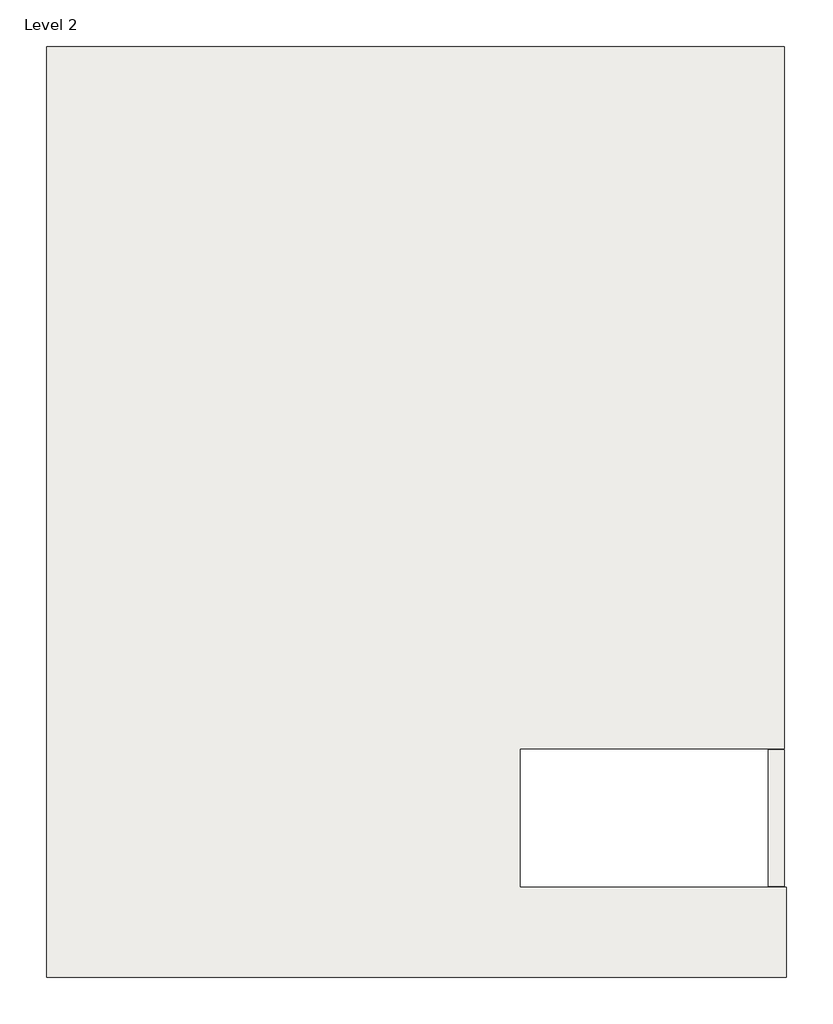
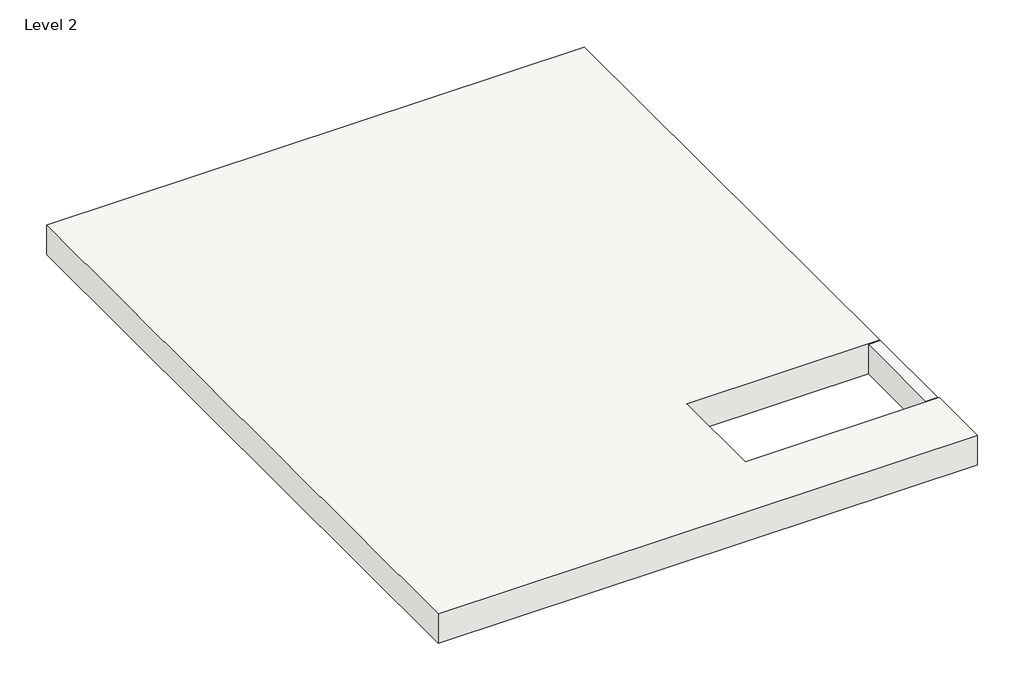
# One storey: 2 roofs.
"""IFC4 building model written with IfcOpenShell, lengths in millimetres."""

from ifc_helpers import new_model, si_unit, frame, origin, place, context, project, spatial, polyline, outline, extrude, element, save

model = new_model("IFC4")

# Units and contexts
model_context = context("Model", 3, world=origin())
ifc_project = project(units=[si_unit("LENGTHUNIT", "METRE", prefix="MILLI")], contexts=[model_context])

# Site, building, storey
site = spatial("IfcSite", under=ifc_project)
building = spatial("IfcBuilding", under=site)
storey = spatial("IfcBuildingStorey", under=building, Name="Level 2", Elevation=3048.0)

# Roofs
placement = place(None, origin())
element("IfcRoof", 1, ObjectType="Steel Truss - Insulation on Metal Deck - EPDM", at=placement, inside=storey, context=model_context, shape_type="SweptSolid", body=[
    extrude(outline(polyline([(-3801.7644177, -1680.1159676), (-3801.7644177, 10105.4840324), (5545.4355823, 10105.4840324), (5545.4355823, 1215.4840324), (2192.6355823, 1215.4840324), (2192.6355823, -537.1159676), (5570.8355823, -537.1159676), (5570.8355823, -1680.1159676), (-3801.7644177, -1680.1159676)])), frame((0.0, 0.0, 3048.0), z_axis=(0.0, 0.0, 1.0), x_axis=(1.0, 0.0, 0.0)), (0.0, 0.0, 1.0), 546.1),
])
element("IfcRoof", 2, ObjectType="Steel Truss - Insulation on Metal Deck - EPDM", at=placement, inside=storey, context=model_context, shape_type="SweptSolid", body=[
    extrude(outline(polyline([(5342.2355823, 1202.7840324), (5545.4355823, 1202.7840324), (5545.4355823, -524.4159676), (5342.2355823, -524.4159676), (5342.2355823, 1202.7840324)])), frame((0.0, 0.0, 3048.0), z_axis=(0.0, 0.0, 1.0), x_axis=(1.0, 0.0, 0.0)), (0.0, 0.0, 1.0), 546.1),
])

save(model, "model.ifc")

# Revit data of these elements
# Type "Steel Truss - Insulation on Metal Deck - EPDM"
#   Assembly Code = "B1020"
#   Layers, outside or top first: 0' - 0 1/4" "Roofing, EPDM Membrane" (function 4); 0' - 5" "Rigid insulation" (function 3); 0' - 0 1/4" "Metal Deck" (function 1); 1' - 4" "Structure, Steel Bar Joist Layer" (function 1)
# Elements 1, 2 (IfcRoof, "Steel Truss - Insulation on Metal Deck - EPDM")
#   built-in parameter 1001705 = 11.7917 (stored number, unit not read)
#   built-in parameter 1001710 = 33615
#   Phase Created = New Construction
#   Materials on its faces: "Structure, Steel Bar Joist Layer", "Roofing, EPDM Membrane"
# Materials
#   "Roofing, EPDM Membrane": class "Generic", colour RGB 127 127 127, transparency 0, Description = "EPDM roof membrane", Cost = 0
#   "Rigid insulation": class "Generic", colour RGB 127 127 127, transparency 0, Description = "Rigid foam insulation board", Cost = 0
#   "Metal Deck": class "Metal", colour RGB 199 199 199, transparency 0, Description = "Steel, mill finish", Cost = 0
#   "Structure, Steel Bar Joist Layer": class "Metal", colour RGB 127 127 127, transparency 0, Description = "Bar joists, thermal airspace", Cost = 0
